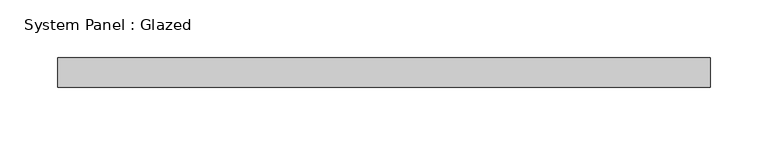
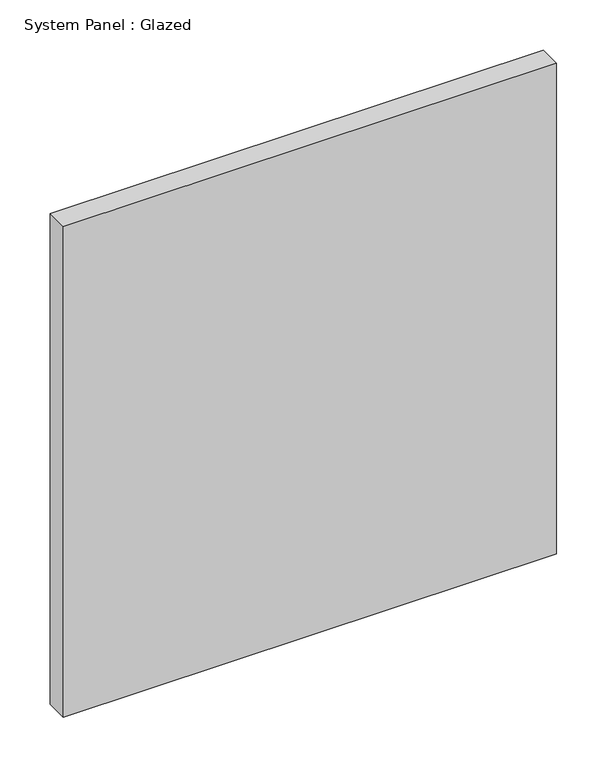
"""IFC4 building model written with IfcOpenShell, lengths in millimetres: plate geometry, System Panel : Glazed."""

from ifc_helpers import new_model, si_unit, origin, origin_with_axes, place, context, project, spatial, polyline, outline, extrude, source, transform, mapped, element, save


def system_panel_glazed_cbb2ce41(model_context):
    return source(origin(), model_context, "Body", "SweptSolid", [
        extrude(outline(polyline([(282.575, 19.05), (-282.575, 19.05), (-282.575, 44.45), (282.575, 44.45), (282.575, 19.05)])), origin_with_axes(), (0.0, 0.0, 1.0), 594.4441631),
    ])


if __name__ == "__main__":
    model = new_model("IFC4")
    model_context = context("Model", 3, world=origin())
    ifc_project = project(units=[si_unit("LENGTHUNIT", "METRE", prefix="MILLI")], contexts=[model_context])
    site = spatial("IfcSite", under=ifc_project)
    building = spatial("IfcBuilding", under=site)
    placement = place(None, origin())
    system_panel_glazed_shape = system_panel_glazed_cbb2ce41(model_context)
    element("IfcPlate", 1, ObjectType="System Panel : Glazed", at=placement, inside=building, context=model_context, shape_type="MappedRepresentation", body=[
        mapped(system_panel_glazed_shape, transform((0.0, 0.0, 0.0), x_axis=(1.0, 0.0, 0.0), y_axis=(0.0, 1.0, 0.0), z_axis=(0.0, 0.0, 1.0))),
    ])
    save(model, "model.ifc")

# Revit data of these elements
# Type "System Panel : Glazed"
#   Construction Type Id = "GSP4R"
#   Analytic Construction = "1/8 in Pilkington single glazing"
#   Visual Light Transmittance = 0.9
#   Solar Heat Gain Coefficient = 0.86
#   Heat Transfer Coefficient (U) = 1.18115 BTU/(h·ft²·°F)
#   Define Thermal Properties by = 1
# Element 1 (IfcPlate, "System Panel : Glazed")
#   Materials on its faces: "Glass"
# Materials
#   "Glass": class "Glass", colour RGB 0 128 192, transparency 0.75, Description = "Soda Lime Glass", Cost = 0
